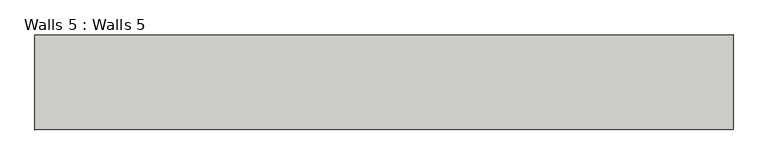
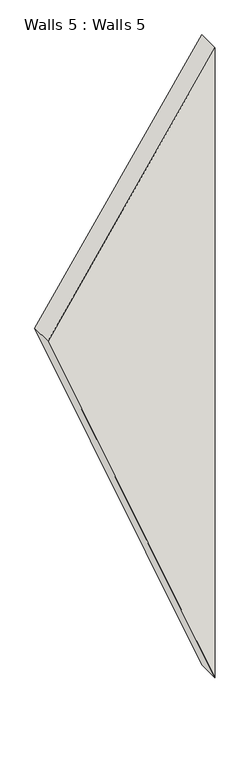
"""IFC4 building model written with IfcOpenShell, lengths in millimetres: wall geometry, Walls 5 : Walls 5."""

from ifc_helpers import new_model, si_unit, frame, origin, place, context, project, spatial, polyline, outline, extrude, source, transform, mapped, element, save


def walls_5_walls_5_14261912(model_context):
    return source(origin(), model_context, "Body", "SweptSolid", [
        extrude(outline(polyline([(0.0, -1871.6311901), (6587.697392, -1871.6311901), (4097.7817636, -3527.2424903), (0.0, -1871.6311901)])), frame((0.0, -4559.9198254, 0.0), z_axis=(0.0, 1.0, 0.0), x_axis=(0.0, 0.0, 1.0)), (0.0, 0.0, 1.0), 225.203632),
    ])


if __name__ == "__main__":
    model = new_model("IFC4")
    model_context = context("Model", 3, world=origin())
    ifc_project = project(units=[si_unit("LENGTHUNIT", "METRE", prefix="MILLI")], contexts=[model_context])
    site = spatial("IfcSite", under=ifc_project)
    building = spatial("IfcBuilding", under=site)
    placement = place(None, origin())
    walls_5_walls_5_shape = walls_5_walls_5_14261912(model_context)
    element("IfcWall", 1, ObjectType="Walls 5 : Walls 5", at=placement, inside=building, context=model_context, shape_type="MappedRepresentation", body=[
        mapped(walls_5_walls_5_shape, transform((0.0, 0.0, 0.0), x_axis=(1.0, 0.0, 0.0), y_axis=(0.0, 1.0, 0.0), z_axis=(0.0, 0.0, 1.0))),
    ])
    save(model, "model.ifc")

# Revit data of these elements
# Element 1 (IfcWall, "Walls 5 : Walls 5")
#   Materials on its faces: "Default Wall"
# Materials
#   "Default Wall": colour RGB 128 128 128, transparency 0
